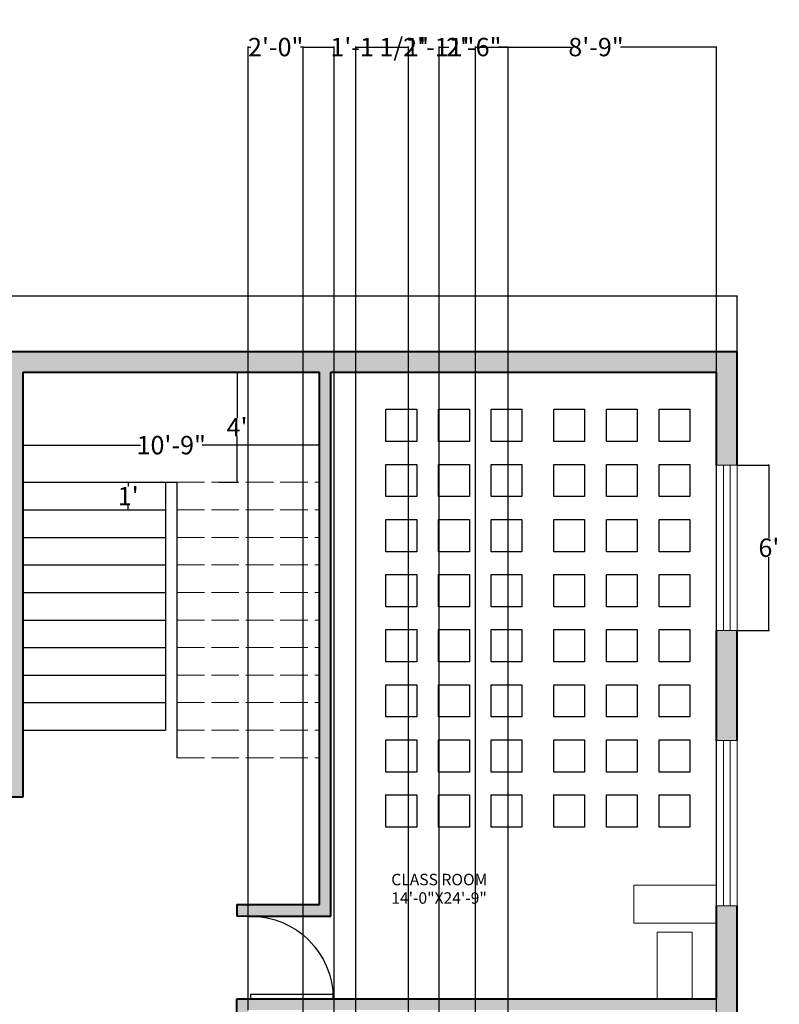
# Model space of a CAD drawing. Units: inches. Extents: x -405 to 940, y 226 to 2032.
# Tile 10 of 10: x 503 to 834, y 1603 to 2032. Entities that reach past the tile are written whole.
import ezdxf

# ---------------------------------------------------------------- set-up
doc = ezdxf.new("R2010")
doc.units = ezdxf.units.IN
doc.header["$MEASUREMENT"] = 0
doc.linetypes.add('ACAD_ISO02W100', pattern=[15, 12, -3])
for name, color, linetype, lineweight in [('A-ANNO-DIMS', 120, 'Continuous', 18), ('A-AREA-IDEN', 32, 'Continuous', 18), ('A-FLOR-STRS-OVHD', 38, 'ACAD_ISO02W100', 18), ('A-FURN-SEAT', 5, 'Continuous', 18), ('A-GLAZ-HIDN', 1, 'ACAD_ISO02W100', 18), ('A-WALL-PATT', 8, 'Continuous', 13), ('door', 6, 'Continuous', 25), ('stair', 38, 'Continuous', 25), ('tables', 2, 'Continuous', 18), ('wall', 3, 'Continuous', 40), ('window', 1, 'Continuous', 18)]:
    doc.layers.add(name, color=color, linetype=linetype, lineweight=lineweight)
doc.layers.add('beches', color=5, linetype='Continuous')
doc.styles.get("Standard").update_dxf_attribs({"font": 'arial.ttf'})
doc.dimstyles.get("Standard").update_dxf_attribs({"dimtxt": 8, "dimasz": 0.18, "dimexe": 0.18, "dimexo": 0.0625, "dimgap": 0.09, "dimtad": 0, "dimtih": 1, "dimtoh": 1, "dimdec": 0, "dimzin": 0, "dimdsep": 46, "dimlunit": 3, "dimtxsty": 'Standard', "dimblk": 'OBLIQUE', "dimcen": 0.09, "dimadec": 0, "dimazin": 0, "dimtfac": 1, "dimtdec": 0, "dimtofl": 0, "dimtmove": 0, "dimatfit": 3, "dimfxl": 1, "dimtolj": 1, "dimtzin": 0, "dimarcsym": 0})

# ---------------------------------------------------------------- blocks, each defined once
blk = doc.blocks.new('*U4')
for p, q in [((0, 0), (0, -6)), ((36, 0), (36, -6))]:
    blk.add_line(p, q)
blk.add_lwpolyline([(0, 0), (0, 36), (1.75, 36), (1.75, 0)], close=True)
blk.add_arc((0, 0), 36, 0, 90)
blk = doc.blocks.new('*U29')
at = {"layer": 'beches'}
blk.add_lwpolyline([(6.71, -7.02), (-6.71, -7.02), (-6.71, 7.02), (6.71, 7.02)], close=True, dxfattribs=at)
blk = doc.blocks.new('*U30')
at = {"layer": 'A-FURN-SEAT', "transparency": 16777216}
for p in [(-45.84, 168), (-45.84, 168, 12), (-45.84, 168, 24), (-45.84, 168, 36), (-45.84, 168, 48), (-45.84, 168, 60), (-45.84, 168, 72), (-45.84, 168, 84), (-45.84, 168, 96), (-45.84, 168, 108), (-45.84, 168, 120), (-45.84, 168, 132), (-22.92, 168), (-22.92, 168, 12), (-22.92, 168, 24), (-22.92, 168, 36), (-22.92, 168, 48), (-22.92, 168, 60), (-22.92, 168, 72), (-22.92, 168, 84), (-22.92, 168, 96), (-22.92, 168, 108), (-22.92, 168, 120), (-22.92, 168, 132), (0, 168), (0, 168, 12), (0, 168, 24), (0, 168, 36), (0, 168, 48), (0, 168, 60), (0, 168, 72), (0, 168, 84), (0, 168, 96), (0, 168, 108), (0, 168, 120), (0, 168, 132), (-45.84, 144), (-45.84, 144, 12), (-45.84, 144, 24), (-45.84, 144, 36), (-45.84, 144, 48), (-45.84, 144, 60), (-45.84, 144, 72), (-45.84, 144, 84), (-45.84, 144, 96), (-45.84, 144, 108), (-45.84, 144, 120), (-45.84, 144, 132), (-22.92, 144), (-22.92, 144, 12), (-22.92, 144, 24), (-22.92, 144, 36), (-22.92, 144, 48), (-22.92, 144, 60), (-22.92, 144, 72), (-22.92, 144, 84), (-22.92, 144, 96), (-22.92, 144, 108), (-22.92, 144, 120), (-22.92, 144, 132), (0, 144), (0, 144, 12), (0, 144, 24), (0, 144, 36), (0, 144, 48), (0, 144, 60), (0, 144, 72), (0, 144, 84), (0, 144, 96), (0, 144, 108), (0, 144, 120), (0, 144, 132), (-45.84, 120), (-45.84, 120, 12), (-45.84, 120, 24), (-45.84, 120, 36), (-45.84, 120, 48), (-45.84, 120, 60), (-45.84, 120, 72), (-45.84, 120, 84), (-45.84, 120, 96), (-45.84, 120, 108), (-45.84, 120, 120), (-45.84, 120, 132), (-22.92, 120), (-22.92, 120, 12), (-22.92, 120, 24), (-22.92, 120, 36), (-22.92, 120, 48), (-22.92, 120, 60), (-22.92, 120, 72), (-22.92, 120, 84), (-22.92, 120, 96), (-22.92, 120, 108), (-22.92, 120, 120), (-22.92, 120, 132), (0, 120), (0, 120, 12), (0, 120, 24), (0, 120, 36), (0, 120, 48), (0, 120, 60), (0, 120, 72), (0, 120, 84), (0, 120, 96), (0, 120, 108), (0, 120, 120), (0, 120, 132), (-45.84, 96), (-45.84, 96, 12), (-45.84, 96, 24), (-45.84, 96, 36), (-45.84, 96, 48), (-45.84, 96, 60), (-45.84, 96, 72), (-45.84, 96, 84), (-45.84, 96, 96), (-45.84, 96, 108), (-45.84, 96, 120), (-45.84, 96, 132), (-22.92, 96), (-22.92, 96, 12), (-22.92, 96, 24), (-22.92, 96, 36), (-22.92, 96, 48), (-22.92, 96, 60), (-22.92, 96, 72), (-22.92, 96, 84), (-22.92, 96, 96), (-22.92, 96, 108), (-22.92, 96, 120), (-22.92, 96, 132), (0, 96), (0, 96, 12), (0, 96, 24), (0, 96, 36), (0, 96, 48), (0, 96, 60), (0, 96, 72), (0, 96, 84), (0, 96, 96), (0, 96, 108), (0, 96, 120), (0, 96, 132), (-45.84, 72), (-45.84, 72, 12), (-45.84, 72, 24), (-45.84, 72, 36), (-45.84, 72, 48), (-45.84, 72, 60), (-45.84, 72, 72), (-45.84, 72, 84), (-45.84, 72, 96), (-45.84, 72, 108), (-45.84, 72, 120), (-45.84, 72, 132), (-22.92, 72), (-22.92, 72, 12), (-22.92, 72, 24), (-22.92, 72, 36), (-22.92, 72, 48), (-22.92, 72, 60), (-22.92, 72, 72), (-22.92, 72, 84), (-22.92, 72, 96), (-22.92, 72, 108), (-22.92, 72, 120), (-22.92, 72, 132), (0, 72), (0, 72, 12), (0, 72, 24), (0, 72, 36), (0, 72, 48), (0, 72, 60), (0, 72, 72), (0, 72, 84), (0, 72, 96), (0, 72, 108), (0, 72, 120), (0, 72, 132), (-45.84, 48), (-45.84, 48, 12), (-45.84, 48, 24), (-45.84, 48, 36), (-45.84, 48, 48), (-45.84, 48, 60), (-45.84, 48, 72), (-45.84, 48, 84), (-45.84, 48, 96), (-45.84, 48, 108), (-45.84, 48, 120), (-45.84, 48, 132), (-22.92, 48), (-22.92, 48, 12), (-22.92, 48, 24), (-22.92, 48, 36), (-22.92, 48, 48), (-22.92, 48, 60), (-22.92, 48, 72), (-22.92, 48, 84), (-22.92, 48, 96), (-22.92, 48, 108), (-22.92, 48, 120), (-22.92, 48, 132), (0, 48), (0, 48, 12), (0, 48, 24), (0, 48, 36), (0, 48, 48), (0, 48, 60), (0, 48, 72), (0, 48, 84), (0, 48, 96), (0, 48, 108), (0, 48, 120), (0, 48, 132), (-45.84, 24), (-45.84, 24, 12), (-45.84, 24, 24), (-45.84, 24, 36), (-45.84, 24, 48), (-45.84, 24, 60), (-45.84, 24, 72), (-45.84, 24, 84), (-45.84, 24, 96), (-45.84, 24, 108), (-45.84, 24, 120), (-45.84, 24, 132), (-22.92, 24), (-22.92, 24, 12), (-22.92, 24, 24), (-22.92, 24, 36), (-22.92, 24, 48), (-22.92, 24, 60), (-22.92, 24, 72), (-22.92, 24, 84), (-22.92, 24, 96), (-22.92, 24, 108), (-22.92, 24, 120), (-22.92, 24, 132), (0, 24), (0, 24, 12), (0, 24, 24), (0, 24, 36), (0, 24, 48), (0, 24, 60), (0, 24, 72), (0, 24, 84), (0, 24, 96), (0, 24, 108), (0, 24, 120), (0, 24, 132), (-45.84, 0), (-45.84, 0, 12), (-45.84, 0, 24), (-45.84, 0, 36), (-45.84, 0, 48), (-45.84, 0, 60), (-45.84, 0, 72), (-45.84, 0, 84), (-45.84, 0, 96), (-45.84, 0, 108), (-45.84, 0, 120), (-45.84, 0, 132), (-22.92, 0), (-22.92, 0, 12), (-22.92, 0, 24), (-22.92, 0, 36), (-22.92, 0, 48), (-22.92, 0, 60), (-22.92, 0, 72), (-22.92, 0, 84), (-22.92, 0, 96), (-22.92, 0, 108), (-22.92, 0, 120), (-22.92, 0, 132), (0, 0), (0, 0, 12), (0, 0, 24), (0, 0, 36), (0, 0, 48), (0, 0, 60), (0, 0, 72), (0, 0, 84), (0, 0, 96), (0, 0, 108), (0, 0, 120), (0, 0, 132)]:
    blk.add_blockref('*U29', p, dxfattribs=at)
blk = doc.blocks.new('*U27')
at = {"layer": 'beches'}
blk.add_lwpolyline([(6.71, -7.02), (-6.71, -7.02), (-6.71, 7.02), (6.71, 7.02)], close=True, dxfattribs=at)
blk = doc.blocks.new('*U28')
at = {"layer": 'A-FURN-SEAT', "transparency": 16777216}
for p in [(-45.84, 168), (-45.84, 168, 12), (-45.84, 168, 24), (-45.84, 168, 36), (-45.84, 168, 48), (-45.84, 168, 60), (-45.84, 168, 72), (-45.84, 168, 84), (-45.84, 168, 96), (-45.84, 168, 108), (-45.84, 168, 120), (-45.84, 168, 132), (-22.92, 168), (-22.92, 168, 12), (-22.92, 168, 24), (-22.92, 168, 36), (-22.92, 168, 48), (-22.92, 168, 60), (-22.92, 168, 72), (-22.92, 168, 84), (-22.92, 168, 96), (-22.92, 168, 108), (-22.92, 168, 120), (-22.92, 168, 132), (0, 168), (0, 168, 12), (0, 168, 24), (0, 168, 36), (0, 168, 48), (0, 168, 60), (0, 168, 72), (0, 168, 84), (0, 168, 96), (0, 168, 108), (0, 168, 120), (0, 168, 132), (-45.84, 144), (-45.84, 144, 12), (-45.84, 144, 24), (-45.84, 144, 36), (-45.84, 144, 48), (-45.84, 144, 60), (-45.84, 144, 72), (-45.84, 144, 84), (-45.84, 144, 96), (-45.84, 144, 108), (-45.84, 144, 120), (-45.84, 144, 132), (-22.92, 144), (-22.92, 144, 12), (-22.92, 144, 24), (-22.92, 144, 36), (-22.92, 144, 48), (-22.92, 144, 60), (-22.92, 144, 72), (-22.92, 144, 84), (-22.92, 144, 96), (-22.92, 144, 108), (-22.92, 144, 120), (-22.92, 144, 132), (0, 144), (0, 144, 12), (0, 144, 24), (0, 144, 36), (0, 144, 48), (0, 144, 60), (0, 144, 72), (0, 144, 84), (0, 144, 96), (0, 144, 108), (0, 144, 120), (0, 144, 132), (-45.84, 120), (-45.84, 120, 12), (-45.84, 120, 24), (-45.84, 120, 36), (-45.84, 120, 48), (-45.84, 120, 60), (-45.84, 120, 72), (-45.84, 120, 84), (-45.84, 120, 96), (-45.84, 120, 108), (-45.84, 120, 120), (-45.84, 120, 132), (-22.92, 120), (-22.92, 120, 12), (-22.92, 120, 24), (-22.92, 120, 36), (-22.92, 120, 48), (-22.92, 120, 60), (-22.92, 120, 72), (-22.92, 120, 84), (-22.92, 120, 96), (-22.92, 120, 108), (-22.92, 120, 120), (-22.92, 120, 132), (0, 120), (0, 120, 12), (0, 120, 24), (0, 120, 36), (0, 120, 48), (0, 120, 60), (0, 120, 72), (0, 120, 84), (0, 120, 96), (0, 120, 108), (0, 120, 120), (0, 120, 132), (-45.84, 96), (-45.84, 96, 12), (-45.84, 96, 24), (-45.84, 96, 36), (-45.84, 96, 48), (-45.84, 96, 60), (-45.84, 96, 72), (-45.84, 96, 84), (-45.84, 96, 96), (-45.84, 96, 108), (-45.84, 96, 120), (-45.84, 96, 132), (-22.92, 96), (-22.92, 96, 12), (-22.92, 96, 24), (-22.92, 96, 36), (-22.92, 96, 48), (-22.92, 96, 60), (-22.92, 96, 72), (-22.92, 96, 84), (-22.92, 96, 96), (-22.92, 96, 108), (-22.92, 96, 120), (-22.92, 96, 132), (0, 96), (0, 96, 12), (0, 96, 24), (0, 96, 36), (0, 96, 48), (0, 96, 60), (0, 96, 72), (0, 96, 84), (0, 96, 96), (0, 96, 108), (0, 96, 120), (0, 96, 132), (-45.84, 72), (-45.84, 72, 12), (-45.84, 72, 24), (-45.84, 72, 36), (-45.84, 72, 48), (-45.84, 72, 60), (-45.84, 72, 72), (-45.84, 72, 84), (-45.84, 72, 96), (-45.84, 72, 108), (-45.84, 72, 120), (-45.84, 72, 132), (-22.92, 72), (-22.92, 72, 12), (-22.92, 72, 24), (-22.92, 72, 36), (-22.92, 72, 48), (-22.92, 72, 60), (-22.92, 72, 72), (-22.92, 72, 84), (-22.92, 72, 96), (-22.92, 72, 108), (-22.92, 72, 120), (-22.92, 72, 132), (0, 72), (0, 72, 12), (0, 72, 24), (0, 72, 36), (0, 72, 48), (0, 72, 60), (0, 72, 72), (0, 72, 84), (0, 72, 96), (0, 72, 108), (0, 72, 120), (0, 72, 132), (-45.84, 48), (-45.84, 48, 12), (-45.84, 48, 24), (-45.84, 48, 36), (-45.84, 48, 48), (-45.84, 48, 60), (-45.84, 48, 72), (-45.84, 48, 84), (-45.84, 48, 96), (-45.84, 48, 108), (-45.84, 48, 120), (-45.84, 48, 132), (-22.92, 48), (-22.92, 48, 12), (-22.92, 48, 24), (-22.92, 48, 36), (-22.92, 48, 48), (-22.92, 48, 60), (-22.92, 48, 72), (-22.92, 48, 84), (-22.92, 48, 96), (-22.92, 48, 108), (-22.92, 48, 120), (-22.92, 48, 132), (0, 48), (0, 48, 12), (0, 48, 24), (0, 48, 36), (0, 48, 48), (0, 48, 60), (0, 48, 72), (0, 48, 84), (0, 48, 96), (0, 48, 108), (0, 48, 120), (0, 48, 132), (-45.84, 24), (-45.84, 24, 12), (-45.84, 24, 24), (-45.84, 24, 36), (-45.84, 24, 48), (-45.84, 24, 60), (-45.84, 24, 72), (-45.84, 24, 84), (-45.84, 24, 96), (-45.84, 24, 108), (-45.84, 24, 120), (-45.84, 24, 132), (-22.92, 24), (-22.92, 24, 12), (-22.92, 24, 24), (-22.92, 24, 36), (-22.92, 24, 48), (-22.92, 24, 60), (-22.92, 24, 72), (-22.92, 24, 84), (-22.92, 24, 96), (-22.92, 24, 108), (-22.92, 24, 120), (-22.92, 24, 132), (0, 24), (0, 24, 12), (0, 24, 24), (0, 24, 36), (0, 24, 48), (0, 24, 60), (0, 24, 72), (0, 24, 84), (0, 24, 96), (0, 24, 108), (0, 24, 120), (0, 24, 132), (-45.84, 0), (-45.84, 0, 12), (-45.84, 0, 24), (-45.84, 0, 36), (-45.84, 0, 48), (-45.84, 0, 60), (-45.84, 0, 72), (-45.84, 0, 84), (-45.84, 0, 96), (-45.84, 0, 108), (-45.84, 0, 120), (-45.84, 0, 132), (-22.92, 0), (-22.92, 0, 12), (-22.92, 0, 24), (-22.92, 0, 36), (-22.92, 0, 48), (-22.92, 0, 60), (-22.92, 0, 72), (-22.92, 0, 84), (-22.92, 0, 96), (-22.92, 0, 108), (-22.92, 0, 120), (-22.92, 0, 132), (0, 0), (0, 0, 12), (0, 0, 24), (0, 0, 36), (0, 0, 48), (0, 0, 60), (0, 0, 72), (0, 0, 84), (0, 0, 96), (0, 0, 108), (0, 0, 120), (0, 0, 132)]:
    blk.add_blockref('*U27', p, dxfattribs=at)
blk = doc.blocks.new('_Oblique')
at = {"color": 0, "linetype": 'ByBlock', "lineweight": -2}
blk.add_line((-0.5, -0.5), (0.5, 0.5), dxfattribs=at)
blk = doc.blocks.new('*D43')
at = {"layer": 'A-ANNO-DIMS', "color": 0, "lineweight": -2, "transparency": 16777216}
for p, q in [((-257.23, 1887.87), (-257.23, 1912.15)), ((-257.23, 1911.97), (265.43, 1911.97)), ((815.77, 1911.97), (293.1, 1911.97)), ((815.77, 1887.87), (815.77, 1912.15))]:
    blk.add_line(p, q, dxfattribs=at)
at = {"layer": 'Defpoints', "color": 0, "transparency": 16777216}
for p in [(815.77, 1911.97), (-257.23, 1887.81), (815.77, 1887.81)]:
    blk.add_point(p, dxfattribs=at)
at = {"layer": 'A-ANNO-DIMS', "color": 0, "lineweight": -2, "transparency": 16777216, "xscale": 0.18, "yscale": 0.18, "zscale": 0.18, "rotation": 180}
blk.add_blockref('_Oblique', (-257.23, 1911.97), dxfattribs=at)
at = {"layer": 'A-ANNO-DIMS', "color": 0, "lineweight": -2, "transparency": 16777216, "xscale": 0.18, "yscale": 0.18, "zscale": 0.18}
blk.add_blockref('_Oblique', (815.77, 1911.97), dxfattribs=at)
at = {"layer": 'A-ANNO-DIMS', "color": 0, "transparency": 16777216, "insert": (279.27, 1911.97), "char_height": 8, "attachment_point": 5}
blk.add_mtext('\\A1;89\'-5"', dxfattribs=at)
blk = doc.blocks.new('*D65')
at = {"layer": 'A-ANNO-DIMS', "color": 0, "lineweight": -2, "transparency": 16777216}
for p, q in [((504.77, 1848.63), (504.77, 1846.83)), ((504.77, 1847.01), (555.81, 1847.01)), ((633.77, 1847.01), (582.72, 1847.01)), ((633.77, 1848.63), (633.77, 1846.83))]:
    blk.add_line(p, q, dxfattribs=at)
at = {"layer": 'Defpoints', "color": 0, "transparency": 16777216}
for p in [(504.77, 1848.69), (633.77, 1848.69), (633.77, 1847.01)]:
    blk.add_point(p, dxfattribs=at)
at = {"layer": 'A-ANNO-DIMS', "color": 0, "lineweight": -2, "transparency": 16777216, "xscale": 0.18, "yscale": 0.18, "zscale": 0.18, "rotation": 180}
blk.add_blockref('_Oblique', (504.77, 1847.01), dxfattribs=at)
at = {"layer": 'A-ANNO-DIMS', "color": 0, "lineweight": -2, "transparency": 16777216, "xscale": 0.18, "yscale": 0.18, "zscale": 0.18}
blk.add_blockref('_Oblique', (633.77, 1847.01), dxfattribs=at)
at = {"layer": 'A-ANNO-DIMS', "color": 0, "transparency": 16777216, "insert": (569.27, 1847.01), "char_height": 8, "attachment_point": 5}
blk.add_mtext('\\A1;10\'-9"', dxfattribs=at)
blk = doc.blocks.new('*D66')
at = {"layer": 'A-ANNO-DIMS', "color": 0, "lineweight": -2, "transparency": 16777216}
for p, q in [((590.05, 1878.81), (598.12, 1878.81)), ((597.94, 1878.81), (597.94, 1858.9)), ((597.94, 1830.81), (597.94, 1850.72)), ((590.05, 1830.81), (598.12, 1830.81))]:
    blk.add_line(p, q, dxfattribs=at)
at = {"layer": 'Defpoints', "color": 0, "transparency": 16777216}
for p in [(589.98, 1878.81), (589.98, 1830.81), (597.94, 1830.81)]:
    blk.add_point(p, dxfattribs=at)
at = {"layer": 'A-ANNO-DIMS', "color": 0, "lineweight": -2, "transparency": 16777216, "xscale": 0.18, "yscale": 0.18, "zscale": 0.18}
for p, rotation in [((597.94, 1878.81), 90), ((597.94, 1830.81), 270)]:
    blk.add_blockref('_Oblique', p, dxfattribs=dict(at, rotation=rotation))
at = {"layer": 'A-ANNO-DIMS', "color": 0, "transparency": 16777216, "insert": (597.94, 1854.81), "char_height": 8, "attachment_point": 5}
blk.add_mtext("\\A1;4'", dxfattribs=at)
blk = doc.blocks.new('*D67')
at = {"layer": 'A-ANNO-DIMS', "color": 0, "lineweight": -2, "transparency": 16777216}
for p, q in [((549.93, 1830.81), (550.72, 1830.81)), ((550.54, 1830.81), (550.54, 1828.92)), ((550.54, 1818.81), (550.54, 1820.7)), ((549.93, 1818.81), (550.72, 1818.81))]:
    blk.add_line(p, q, dxfattribs=at)
at = {"layer": 'Defpoints', "color": 0, "transparency": 16777216}
for p in [(549.87, 1830.81), (549.87, 1818.81), (550.54, 1818.81)]:
    blk.add_point(p, dxfattribs=at)
at = {"layer": 'A-ANNO-DIMS', "color": 0, "lineweight": -2, "transparency": 16777216, "xscale": 0.18, "yscale": 0.18, "zscale": 0.18}
for p, rotation in [((550.54, 1830.81), 90), ((550.54, 1818.81), 270)]:
    blk.add_blockref('_Oblique', p, dxfattribs=dict(at, rotation=rotation))
at = {"layer": 'A-ANNO-DIMS', "color": 0, "transparency": 16777216, "insert": (550.54, 1824.81), "char_height": 8, "attachment_point": 5}
blk.add_mtext("\\A1;1'", dxfattribs=at)
blk = doc.blocks.new('*D68')
at = {"layer": 'A-ANNO-DIMS', "color": 0, "lineweight": -2, "transparency": 16777216}
for p, q in [((815.83, 1838.31), (829.73, 1838.31)), ((829.55, 1838.31), (829.55, 1806.48)), ((829.55, 1766.31), (829.55, 1798.14)), ((815.83, 1766.31), (829.73, 1766.31))]:
    blk.add_line(p, q, dxfattribs=at)
at = {"layer": 'Defpoints', "color": 0, "transparency": 16777216}
for p in [(815.77, 1838.31), (815.77, 1766.31), (829.55, 1766.31)]:
    blk.add_point(p, dxfattribs=at)
at = {"layer": 'A-ANNO-DIMS', "color": 0, "lineweight": -2, "transparency": 16777216, "xscale": 0.18, "yscale": 0.18, "zscale": 0.18}
for p, rotation in [((829.55, 1838.31), 90), ((829.55, 1766.31), 270)]:
    blk.add_blockref('_Oblique', p, dxfattribs=dict(at, rotation=rotation))
at = {"layer": 'A-ANNO-DIMS', "color": 0, "transparency": 16777216, "insert": (829.55, 1802.31), "char_height": 8, "attachment_point": 5}
blk.add_mtext("\\A1;6'", dxfattribs=at)
blk = doc.blocks.new('CHAIR-DESK')
blk.add_lwpolyline([(0, 15.21), (28.97, 15.21), (28.97, 0), (0, 0)], close=True)
blk = doc.blocks.new('WIN-PANE-72IN')
for p, q in [((0, 3), (72, 3)), ((0, 0), (72, 0))]:
    blk.add_line(p, q)
blk = doc.blocks.new('*D99')
at = {"layer": 'A-ANNO-DIMS', "color": 0, "lineweight": -2, "transparency": 16777216}
for p, q in [((626.77, 1569.91), (626.77, 2020.64)), ((626.77, 2020.46), (640.19, 2020.46)), ((640.19, 1569.91), (640.19, 2020.64)), ((640.19, 2020.46), (640.37, 2020.46))]:
    blk.add_line(p, q, dxfattribs=at)
at = {"layer": 'Defpoints', "color": 0, "transparency": 16777216}
for p in [(640.19, 2020.46), (626.77, 1569.84), (640.19, 1569.84)]:
    blk.add_point(p, dxfattribs=at)
at = {"layer": 'A-ANNO-DIMS', "color": 0, "lineweight": -2, "transparency": 16777216, "xscale": 0.18, "yscale": 0.18, "zscale": 0.18, "rotation": 180}
blk.add_blockref('_Oblique', (626.77, 2020.46), dxfattribs=at)
at = {"layer": 'A-ANNO-DIMS', "color": 0, "lineweight": -2, "transparency": 16777216, "xscale": 0.18, "yscale": 0.18, "zscale": 0.18}
blk.add_blockref('_Oblique', (640.19, 2020.46), dxfattribs=at)
at = {"layer": 'A-ANNO-DIMS', "color": 0, "transparency": 16777216, "insert": (660.04, 2020.46), "char_height": 8, "attachment_point": 5}
blk.add_mtext('\\A1;1\'-1 1/2"', dxfattribs=at)
blk = doc.blocks.new('*D101')
at = {"layer": 'A-ANNO-DIMS', "color": 0, "lineweight": -2, "transparency": 16777216}
for p, q in [((649.69, 1569.91), (649.69, 2020.64)), ((649.69, 2020.46), (672.61, 2020.46)), ((672.61, 1569.91), (672.61, 2020.64)), ((672.61, 2020.46), (672.79, 2020.46))]:
    blk.add_line(p, q, dxfattribs=at)
at = {"layer": 'Defpoints', "color": 0, "transparency": 16777216}
for p in [(672.61, 2020.46), (649.69, 1569.84), (672.61, 1569.84)]:
    blk.add_point(p, dxfattribs=at)
at = {"layer": 'A-ANNO-DIMS', "color": 0, "lineweight": -2, "transparency": 16777216, "xscale": 0.18, "yscale": 0.18, "zscale": 0.18, "rotation": 180}
blk.add_blockref('_Oblique', (649.69, 2020.46), dxfattribs=at)
at = {"layer": 'A-ANNO-DIMS', "color": 0, "lineweight": -2, "transparency": 16777216, "xscale": 0.18, "yscale": 0.18, "zscale": 0.18}
blk.add_blockref('_Oblique', (672.61, 2020.46), dxfattribs=at)
at = {"layer": 'A-ANNO-DIMS', "color": 0, "transparency": 16777216, "insert": (686.25, 2020.46), "char_height": 8, "attachment_point": 5}
blk.add_mtext('\\A1;1\'-11"', dxfattribs=at)
blk = doc.blocks.new('*D103')
at = {"layer": 'A-ANNO-DIMS', "color": 0, "lineweight": -2, "transparency": 16777216}
for p, q in [((686.03, 1569.91), (686.03, 2020.64)), ((686.03, 2020.46), (690.24, 2020.46)), ((716.03, 2020.46), (711.82, 2020.46)), ((716.03, 1569.91), (716.03, 2020.64))]:
    blk.add_line(p, q, dxfattribs=at)
at = {"layer": 'Defpoints', "color": 0, "transparency": 16777216}
for p in [(716.03, 2020.46), (686.03, 1569.84), (716.03, 1569.84)]:
    blk.add_point(p, dxfattribs=at)
at = {"layer": 'A-ANNO-DIMS', "color": 0, "lineweight": -2, "transparency": 16777216, "xscale": 0.18, "yscale": 0.18, "zscale": 0.18, "rotation": 180}
blk.add_blockref('_Oblique', (686.03, 2020.46), dxfattribs=at)
at = {"layer": 'A-ANNO-DIMS', "color": 0, "lineweight": -2, "transparency": 16777216, "xscale": 0.18, "yscale": 0.18, "zscale": 0.18}
blk.add_blockref('_Oblique', (716.03, 2020.46), dxfattribs=at)
at = {"layer": 'A-ANNO-DIMS', "color": 0, "transparency": 16777216, "insert": (701.03, 2020.46), "char_height": 8, "attachment_point": 5}
blk.add_mtext('\\A1;2\'-6"', dxfattribs=at)
blk = doc.blocks.new('*D104')
at = {"layer": 'A-ANNO-DIMS', "color": 0, "lineweight": -2, "transparency": 16777216}
for p, q in [((602.77, 1600.87), (602.77, 2020.64)), ((602.77, 2020.46), (603.98, 2020.46)), ((626.77, 2020.46), (625.56, 2020.46)), ((626.77, 1569.91), (626.77, 2020.64))]:
    blk.add_line(p, q, dxfattribs=at)
at = {"layer": 'Defpoints', "color": 0, "transparency": 16777216}
for p in [(626.77, 2020.46), (602.77, 1600.81), (626.77, 1569.84)]:
    blk.add_point(p, dxfattribs=at)
at = {"layer": 'A-ANNO-DIMS', "color": 0, "lineweight": -2, "transparency": 16777216, "xscale": 0.18, "yscale": 0.18, "zscale": 0.18, "rotation": 180}
blk.add_blockref('_Oblique', (602.77, 2020.46), dxfattribs=at)
at = {"layer": 'A-ANNO-DIMS', "color": 0, "lineweight": -2, "transparency": 16777216, "xscale": 0.18, "yscale": 0.18, "zscale": 0.18}
blk.add_blockref('_Oblique', (626.77, 2020.46), dxfattribs=at)
at = {"layer": 'A-ANNO-DIMS', "color": 0, "transparency": 16777216, "insert": (614.77, 2020.46), "char_height": 8, "attachment_point": 5}
blk.add_mtext('\\A1;2\'-0"', dxfattribs=at)
blk = doc.blocks.new('*D112')
at = {"layer": 'A-ANNO-DIMS', "color": 0, "lineweight": -2, "transparency": 16777216}
for p, q in [((701.77, 534.87), (701.77, 2020.64)), ((701.77, 2020.46), (743.54, 2020.46)), ((806.77, 2020.46), (765, 2020.46)), ((806.77, 534.87), (806.77, 2020.64))]:
    blk.add_line(p, q, dxfattribs=at)
at = {"layer": 'Defpoints', "color": 0, "transparency": 16777216}
for p in [(701.77, 2020.46), (701.77, 534.81), (806.77, 534.81)]:
    blk.add_point(p, dxfattribs=at)
at = {"layer": 'A-ANNO-DIMS', "color": 0, "lineweight": -2, "transparency": 16777216, "xscale": 0.18, "yscale": 0.18, "zscale": 0.18, "rotation": 180}
blk.add_blockref('_Oblique', (701.77, 2020.46), dxfattribs=at)
at = {"layer": 'A-ANNO-DIMS', "color": 0, "lineweight": -2, "transparency": 16777216, "xscale": 0.18, "yscale": 0.18, "zscale": 0.18}
blk.add_blockref('_Oblique', (806.77, 2020.46), dxfattribs=at)
at = {"layer": 'A-ANNO-DIMS', "color": 0, "transparency": 16777216, "insert": (754.27, 2020.46), "char_height": 8, "attachment_point": 5}
blk.add_mtext('\\A1;8\'-9"', dxfattribs=at)

msp = doc.modelspace()

# ---------------------------------------------------------------- hatches: boundary and pattern name
at = {"layer": 'A-WALL-PATT'}
h = msp.add_hatch(dxfattribs=at)
h.set_pattern_fill('AR-HBONE', color=256)
h.set_pattern_definition([(45, (599.8442, 904.9158), (0, 5.656854), [12, -4]), (135, (602.6726, 907.744), (4e-16, 5.656854), [12, -4])])
h.paths.add_polyline_path([(-248.23, 1045.81), (-257.23, 1045.81), (-257.23, 964.81), (-248.23, 964.81)], flags=17)
h.paths.add_polyline_path([(-248.23, 851.81), (-39.23, 851.81), (-39.23, 856.81), (-44.23, 856.81), (-248.23, 856.81), (-248.23, 892.81), (-257.23, 892.81), (-257.23, 839.81), (-248.23, 839.81)])
h.paths.add_polyline_path([(-248.23, 750.81), (124.74, 750.81), (124.74, 751.73), (124.74, 755.81), (-248.23, 755.81), (-248.23, 767.81), (-257.23, 767.81), (-257.23, 726.81), (-248.23, 726.81)])
h.paths.add_polyline_path([(-248.23, 654.81), (-257.23, 654.81), (-257.23, 630.81), (-248.23, 630.81)])
h.paths.add_polyline_path([(-180.23, 534.81), (-248.23, 534.81), (-248.23, 558.81), (-257.23, 558.81), (-257.23, 525.81), (-180.23, 525.81)])
h.paths.add_polyline_path([(-69.23, 534.81), (-108.23, 534.81), (-108.23, 525.81), (-69.23, 525.81)])
h.paths.add_polyline_path([(35.77, 534.81), (2.77, 534.81), (2.77, 525.81), (35.77, 525.81)])
h.paths.add_polyline_path([(182.77, 755.81), (160.74, 755.81), (160.74, 750.81), (177.77, 750.81), (177.77, 534.81), (107.77, 534.81), (107.77, 525.81), (182.77, 525.81)])
h.paths.add_polyline_path([(-39.23, 1609.81), (-44.23, 1609.81), (-44.23, 1604.81), (-44.23, 1460.81), (-135.23, 1460.81), (-135.23, 1465.73), (-140.23, 1465.73), (-140.23, 1460.81), (-248.23, 1460.81), (-248.23, 1471.31), (-257.23, 1471.31), (-257.23, 1419.81), (-248.23, 1419.81), (-248.23, 1455.81), (-44.23, 1455.81), (-44.23, 1194.81), (-39.23, 1194.81)])
h.paths.add_polyline_path([(-248.23, 1520.81), (-257.23, 1520.81), (-257.23, 1495.31), (-248.23, 1495.31), (-248.23, 1505.81), (-140.23, 1505.81), (-140.23, 1495.73), (-135.23, 1495.73), (-135.23, 1516.79), (-140.23, 1516.79), (-140.23, 1510.81), (-248.23, 1510.81)], flags=17)
h.paths.add_polyline_path([(-248.23, 1570.31), (-257.23, 1570.31), (-257.23, 1544.81), (-248.23, 1544.81), (-248.23, 1554.81), (-140.23, 1554.81), (-140.23, 1546.79), (-135.23, 1546.79), (-135.23, 1565.08), (-140.23, 1565.08), (-140.23, 1559.81), (-248.23, 1559.81)], flags=17)
h.paths.add_polyline_path([(-248.23, 1615.81), (-257.23, 1615.81), (-257.23, 1594.31), (-248.23, 1594.31), (-248.23, 1604.81), (-140.23, 1604.81), (-140.23, 1595.08), (-135.23, 1595.08), (-135.23, 1604.81), (-80.23, 1604.81), (-80.23, 1609.81), (-248.23, 1609.81)])
h.paths.add_polyline_path([(-248.23, 1783.81), (-235.46, 1783.81), (-235.46, 1788.81), (-248.23, 1788.81), (-248.23, 1878.81), (-237.73, 1878.81), (-237.73, 1887.81), (-257.23, 1887.81), (-257.23, 1687.81), (-248.23, 1687.81), (-248.23, 1693.81), (-136.23, 1693.81), (-136.23, 1698.81), (-248.23, 1698.81)])
h.paths.add_polyline_path([(-188.23, 1887.81), (-213.73, 1887.81), (-213.73, 1878.81), (-203.23, 1878.81), (-203.23, 1788.81), (-205.46, 1788.81), (-205.46, 1783.81), (-186.39, 1783.81), (-186.39, 1788.81), (-198.23, 1788.81), (-198.23, 1878.81), (-188.23, 1878.81)])
h.paths.add_polyline_path([(-139.23, 1887.81), (-164.23, 1887.81), (-164.23, 1878.81), (-154.23, 1878.81), (-154.23, 1788.81), (-156.39, 1788.81), (-156.39, 1783.81), (-138.25, 1783.81), (-138.25, 1788.81), (-149.23, 1788.81), (-149.23, 1878.81), (-139.23, 1878.81)])
h.paths.add_polyline_path([(-89.23, 1887.81), (-115.23, 1887.81), (-115.23, 1878.81), (-105.23, 1878.81), (-105.23, 1788.81), (-108.25, 1788.81), (-108.25, 1783.81), (-86.45, 1783.81), (-86.45, 1788.81), (-100.23, 1788.81), (-100.23, 1878.81), (-89.23, 1878.81)])
h.paths.add_polyline_path([(-36.23, 1887.81), (-65.23, 1887.81), (-65.23, 1878.81), (-54.23, 1878.81), (-54.23, 1788.81), (-56.45, 1788.81), (-56.45, 1783.81), (-54.23, 1783.81), (-54.23, 1698.81), (-100.23, 1698.81), (-100.23, 1693.81), (-49.23, 1693.81), (-49.23, 1698.81), (-49.23, 1878.81), (-36.23, 1878.81)])
h.paths.add_polyline_path([(89.77, 1887.81), (35.77, 1887.81), (35.77, 1878.81), (48.77, 1878.81), (48.77, 1698.81), (-13.23, 1698.81), (-13.23, 1693.81), (53.77, 1693.81), (53.77, 1698.81), (53.77, 1878.81), (89.77, 1878.81)])
h.paths.add_polyline_path([(255.27, 1887.81), (161.77, 1887.81), (161.77, 1878.81), (197.77, 1878.81), (197.77, 1698.81), (89.77, 1698.81), (89.77, 1693.81), (202.77, 1693.81), (202.77, 1698.81), (202.77, 1878.81), (255.27, 1878.81)])
h.paths.add_polyline_path([(375.27, 1887.81), (327.27, 1887.81), (327.27, 1878.81), (375.27, 1878.81)], flags=17)
h.paths.add_polyline_path([(815.77, 1887.81), (447.27, 1887.81), (447.27, 1878.81), (499.77, 1878.81), (499.77, 1698.81), (238.77, 1698.81), (238.77, 1693.81), (504.77, 1693.81), (504.77, 1878.81), (633.77, 1878.81), (633.77, 1646.81), (597.77, 1646.81), (597.77, 1641.81), (602.77, 1641.81), (638.77, 1641.81), (638.77, 1878.81), (806.77, 1878.81), (806.77, 1838.31), (815.77, 1838.31)])
h.paths.add_polyline_path([(815.77, 1766.31), (806.77, 1766.31), (806.77, 1718.31), (815.77, 1718.31)], flags=17)
h.paths.add_polyline_path([(815.77, 1356.31), (806.77, 1356.31), (806.77, 1303.81), (602.77, 1303.81), (597.77, 1303.81), (597.77, 1037.81), (602.77, 1037.81), (602.77, 1298.81), (806.77, 1298.81), (806.77, 1246.31), (815.77, 1246.31)])
h.paths.add_polyline_path([(815.77, 1174.31), (806.77, 1174.31), (806.77, 1126.31), (815.77, 1126.31)], flags=17)
h.paths.add_polyline_path([(815.77, 1054.31), (806.77, 1054.31), (806.77, 1001.81), (796.08, 1001.81), (796.08, 1001.75), (780.86, 1001.75), (602.77, 1001.81), (597.77, 1001.81), (597.77, 892.81), (602.77, 892.81), (602.77, 996.81), (806.77, 996.81), (806.77, 962.81), (815.77, 962.81)])
h.paths.add_polyline_path([(403.77, 534.81), (379.77, 534.81), (379.77, 525.81), (403.77, 525.81)])
h.paths.add_polyline_path([(-39.23, 1158.81), (-44.23, 1158.81), (-248.23, 1158.81), (-248.23, 1194.81), (-257.23, 1194.81), (-257.23, 1117.81), (-248.23, 1117.81), (-248.23, 1153.81), (-44.23, 1153.81), (-44.23, 892.81), (-39.23, 892.81)])
h.paths.add_polyline_path([(-248.23, 1347.81), (-257.23, 1347.81), (-257.23, 1275.81), (-248.23, 1275.81)], flags=17)
h.paths.add_polyline_path([(815.77, 1476.31), (806.77, 1476.31), (806.77, 1428.31), (815.77, 1428.31)], flags=17)
h.paths.add_polyline_path([(815.77, 1646.31), (806.77, 1646.31), (806.77, 1638.65), (806.77, 1605.81), (597.77, 1605.81), (597.77, 1339.81), (602.77, 1339.81), (602.77, 1600.81), (806.77, 1600.81), (806.77, 1548.31), (815.77, 1548.31)])

# ---------------------------------------------------------------- linework, layer by layer
at = {"layer": 'A-FLOR-STRS-OVHD'}
for p, q in [((571.77, 1830.81), (633.77, 1830.81)), ((571.77, 1818.81), (633.77, 1818.81)), ((571.77, 1806.81), (633.77, 1806.81)), ((571.77, 1794.81), (633.77, 1794.81)), ((571.77, 1782.81), (633.77, 1782.81)), ((571.77, 1770.81), (633.77, 1770.81)), ((571.77, 1758.81), (633.77, 1758.81)), ((571.77, 1746.81), (633.77, 1746.81)), ((571.77, 1734.81), (633.77, 1734.81)), ((571.77, 1722.81), (633.77, 1722.81)), ((571.77, 1710.81), (633.77, 1710.81))]:
    msp.add_line(p, q, dxfattribs=at)
at = {"layer": 'A-GLAZ-HIDN'}
for p, q in [((806.77, 1838.31), (815.77, 1838.31)), ((806.77, 1766.31), (815.77, 1766.31)), ((806.77, 1718.31), (815.77, 1718.31)), ((806.77, 1646.31), (815.77, 1646.31))]:
    msp.add_line(p, q, dxfattribs=at)
at = {"layer": 'door'}
for p, q in [((597.77, 1641.81), (602.77, 1641.81)), ((597.77, 1605.81), (602.77, 1605.81))]:
    msp.add_line(p, q, dxfattribs=at)
at = {"layer": 'stair'}
for p, q in [((504.77, 1830.81), (571.77, 1830.81)), ((566.77, 1830.81), (566.77, 1722.81)), ((571.77, 1830.81), (571.77, 1710.81)), ((504.77, 1818.81), (566.77, 1818.81)), ((504.77, 1806.81), (566.77, 1806.81)), ((504.77, 1794.81), (566.77, 1794.81)), ((504.77, 1782.81), (566.77, 1782.81)), ((504.77, 1770.81), (566.77, 1770.81)), ((504.77, 1758.81), (566.77, 1758.81)), ((504.77, 1746.81), (566.77, 1746.81)), ((504.77, 1734.81), (566.77, 1734.81)), ((504.77, 1722.81), (566.77, 1722.81))]:
    msp.add_line(p, q, dxfattribs=at)
at = {"layer": 'tables'}
for p, q in [((770.77, 1638.65), (770.77, 1655.22)), ((770.77, 1655.22), (806.77, 1655.22)), ((806.77, 1655.22), (806.77, 1638.65)), ((806.77, 1638.65), (770.77, 1638.65))]:
    msp.add_line(p, q, dxfattribs=at)
at = {"layer": 'wall'}
for p, q in [((447.27, 1887.81), (815.77, 1887.81)), ((815.77, 1838.31), (815.77, 1887.81)), ((504.77, 1693.81), (504.77, 1878.81)), ((504.77, 1878.81), (633.77, 1878.81)), ((633.77, 1646.81), (633.77, 1878.81)), ((638.77, 1641.81), (638.77, 1878.81)), ((638.77, 1878.81), (806.77, 1878.81)), ((806.77, 1838.31), (806.77, 1878.81)), ((806.77, 1718.31), (806.77, 1766.31)), ((815.77, 1718.31), (815.77, 1766.31)), ((238.77, 1693.81), (504.77, 1693.81)), ((597.77, 1646.81), (633.77, 1646.81)), ((597.77, 1646.81), (597.77, 1641.81)), ((806.77, 1605.81), (806.77, 1646.31)), ((815.77, 1548.31), (815.77, 1646.31)), ((602.77, 1641.81), (638.77, 1641.81)), ((597.77, 1605.81), (806.77, 1605.81)), ((597.77, 1339.81), (597.77, 1605.81))]:
    msp.add_line(p, q, dxfattribs=at)
at = {"layer": 'window'}
for p, q in [((806.77, 1838.31), (806.77, 1766.31)), ((815.77, 1838.31), (815.77, 1766.31)), ((806.77, 1718.31), (806.77, 1646.31)), ((815.77, 1718.31), (815.77, 1646.31))]:
    msp.add_line(p, q, dxfattribs=at)

# ---------------------------------------------------------------- block references
at = {"layer": 'A-FURN-SEAT'}
for name, p in [('*U28', (715.32, 1687.59)), ('*U30', (788.44, 1687.59))]:
    msp.add_blockref(name, p, dxfattribs=at)
at = {"layer": 'A-FURN-SEAT', "rotation": 90.0000000000003}
msp.add_blockref('CHAIR-DESK', (796.08, 1605.81), dxfattribs=at)
at = {"layer": 'door', "xscale": -1, "rotation": 270}
msp.add_blockref('*U4', (603.77, 1605.81), dxfattribs=at)
at = {"layer": 'window', "rotation": 90.00000000000018}
for p in [(812.77, 1766.31), (812.77, 1646.31)]:
    msp.add_blockref('WIN-PANE-72IN', p, dxfattribs=at)

# ---------------------------------------------------------------- texts
at = {"layer": 'A-AREA-IDEN'}
for s, p in [('CLASS ROOM ', (665.1, 1655.21)), ('14\'-0"X24\'-9"', (665.1, 1647.18))]:
    msp.add_text(s, height=5, dxfattribs=at).set_placement(p)

# ---------------------------------------------------------------- dimensions: what is measured, and where the dimension line sits
at = {"layer": 'A-ANNO-DIMS'}
for base, p1, p2, override, picture, middle in [((640.19, 2020.46), (626.77, 1569.84), (640.19, 1569.84), {"dimdec": 1, "dimlfac": 1, "dimrnd": 0, "dimzin": 1, "dimdsep": 46, "dimlunit": 4, "dimfrac": 2}, '*D99', (660.04, 2020.46)), ((626.77, 2020.46), (602.77, 1600.81), (626.77, 1569.84), {"dimdec": 1, "dimlfac": 1, "dimrnd": 0, "dimzin": 1, "dimdsep": 46, "dimlunit": 4, "dimfrac": 2}, '*D104', (614.77, 2020.46)), ((672.61, 2020.46), (649.69, 1569.84), (672.61, 1569.84), {"dimdec": 1, "dimlfac": 1, "dimrnd": 0, "dimzin": 1, "dimdsep": 46, "dimlunit": 4, "dimfrac": 2}, '*D101', (686.25, 2020.46)), ((716.03, 2020.46), (686.03, 1569.84), (716.03, 1569.84), {"dimdec": 1, "dimlfac": 1, "dimrnd": 0, "dimzin": 1, "dimdsep": 46, "dimlunit": 4, "dimfrac": 2}, '*D103', (701.03, 2020.46)), ((701.77, 2020.46), (806.77, 534.81), (701.77, 534.81), {"dimdec": 1, "dimlfac": 1, "dimrnd": 0, "dimzin": 1, "dimdsep": 46, "dimlunit": 4, "dimfrac": 2}, '*D112', (754.27, 2020.46)), ((815.77, 1911.97), (-257.23, 1887.81), (815.77, 1887.81), {"dimclrd": 0, "dimclre": 0, "dimclrt": 0}, '*D43', (279.27, 1911.97)), ((633.77, 1847.01), (504.77, 1848.69), (633.77, 1848.69), {"dimclrd": 0, "dimclre": 0, "dimclrt": 0}, '*D65', (569.27, 1847.01))]:
    dim = msp.add_linear_dim(base=base, p1=p1, p2=p2, dimstyle='Standard', override=override, dxfattribs=at)
    dim.commit()
    dim.dimension.update_dxf_attribs({"geometry": picture, "text_midpoint": middle})
for base, p1, p2, picture, middle in [((597.94, 1830.81), (589.98, 1878.81), (589.98, 1830.81), '*D66', (597.94, 1854.81)), ((829.55, 1766.31), (815.77, 1838.31), (815.77, 1766.31), '*D68', (829.55, 1802.31)), ((550.54, 1818.81), (549.87, 1830.81), (549.87, 1818.81), '*D67', (550.54, 1824.81))]:
    dim = msp.add_linear_dim(base=base, p1=p1, p2=p2, angle=90, dimstyle='Standard', override={"dimclrd": 0, "dimclre": 0, "dimclrt": 0}, dxfattribs=at)
    dim.commit()
    dim.dimension.update_dxf_attribs({"geometry": picture, "text_midpoint": middle})

doc.saveas('drawing.dxf')
